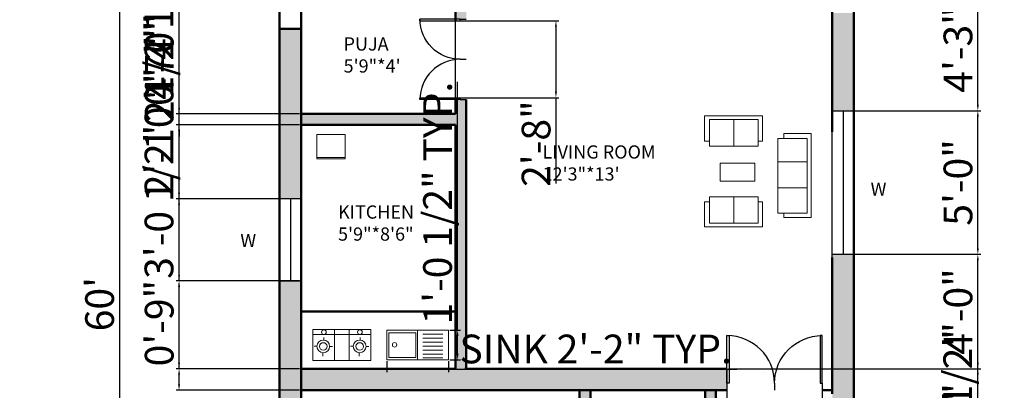
# Model space of a CAD drawing. Units: inches. Extents: x 2063 to 3370, y 2091 to 2971.
# Tile 8 of 14: x 2494 to 2906, y 2468 to 2623. Entities that reach past the tile are written whole.
import ezdxf

# ---------------------------------------------------------------- set-up
doc = ezdxf.new("R2010")
doc.units = ezdxf.units.IN
for name, color, linetype, lineweight in [('A-ANNO-DIMS', 2, 'Continuous', 18), ('A-ANNO-TEXT', 7, 'Continuous', 18), ('A-AREA-IDEN', 3, 'Continuous', 18), ('A-COLS', 7, 'Continuous', 50), ('A-DOOR', 4, 'Continuous', 25), ('A-EQPM', 8, 'Continuous', 18), ('A-FLOR-FIXT', 9, 'Continuous', 18), ('A-FURN', 8, 'Continuous', 18), ('A-GLAZ', 131, 'Continuous', 25), ('A-WALL', 7, 'Continuous', 50), ('A-WALL-PATT', 8, 'Continuous', 13)]:
    doc.layers.add(name, color=color, linetype=linetype, lineweight=lineweight)
doc.styles.get("Standard").update_dxf_attribs({"font": 'arial.ttf'})
doc.dimstyles.new('ISO-25', dxfattribs={"dimtxt": 12, "dimasz": 2.5, "dimexe": 1.25, "dimexo": 0.625, "dimtad": 1, "dimdec": 0, "dimlunit": 4, "dimtxsty": 'Standard', "dimcen": 2.5, "dimadec": 0, "dimazin": 0, "dimtfac": 1, "dimtdec": 0, "dimtmove": 0, "dimatfit": 3, "dimfxl": 1, "dimarcsym": 0})

# ---------------------------------------------------------------- blocks, each defined once
blk = doc.blocks.new('*D8')
at = {"layer": 'A-ANNO-DIMS', "color": 0, "lineweight": -2, "transparency": 16777216}
for p, q in [((2602.12, 2864.43), (2534.59, 2864.43)), ((2535.84, 2861.93), (2535.84, 2146.93)), ((2602.12, 2144.43), (2534.59, 2144.43))]:
    blk.add_line(p, q, dxfattribs=at)
at = {"layer": 'A-ANNO-DIMS', "color": 0, "transparency": 16777216}
for points in [[(2535.42, 2861.93), (2536.25, 2861.93), (2535.84, 2864.43)], [(2535.42, 2146.93), (2536.25, 2146.93), (2535.84, 2144.43)]]:
    blk.add_solid(points, dxfattribs=at)
at = {"layer": 'Defpoints', "color": 0, "transparency": 16777216}
for p in [(2602.75, 2864.43), (2535.84, 2144.43), (2602.75, 2144.43)]:
    blk.add_point(p, dxfattribs=at)
at = {"layer": 'A-ANNO-DIMS', "color": 0, "transparency": 16777216, "insert": (2529.08, 2504.43), "char_height": 12, "attachment_point": 5, "rotation": 90}
blk.add_mtext("60'", dxfattribs=at)
blk = doc.blocks.new('*U2')
for p, q in [((0, 0), (0, -6)), ((40, 0), (40, -6))]:
    blk.add_line(p, q)
blk.add_lwpolyline([(0, 0), (0, 40), (1.75, 40), (1.75, 0)], close=True)
blk.add_arc((0, 0), 40, 0, 90)
blk = doc.blocks.new('SOFA-2SEAT')
for p, q in [((0, 2.07), (0, 12.63)), ((0, 12.63), (24.16, 12.63)), ((24.16, 12.63), (24.16, 2.07)), ((12.27, 11.03), (12.27, 0)), ((2.08, 2.07), (0, 2.07)), ((24.16, 2.07), (22.46, 2.07))]:
    blk.add_line(p, q)
blk.add_lwpolyline([(22.46, 0), (2.08, 0), (2.08, 11.03), (22.46, 11.03)], close=True)
blk = doc.blocks.new('SOFA-3SEAT')
for p, q in [((2.4, 33.13), (2.4, 35.12)), ((2.4, 35.12), (13.91, 35.12)), ((13.91, 35.12), (13.91, 0)), ((0, 23.31), (12.18, 23.31)), ((0, 12.42), (12.18, 12.42)), ((2.4, 0), (2.4, 1.81)), ((13.91, 0), (2.4, 0))]:
    blk.add_line(p, q)
blk.add_lwpolyline([(12.18, 33.13), (0, 33.13), (0, 1.81), (12.18, 1.81)], close=True)
blk = doc.blocks.new('SINK')
for p, q in [((12.88, 12.38), (12.88, 0)), ((15.15, 10.72), (23.41, 10.72)), ((15.15, 9.06), (23.41, 9.06)), ((15.15, 7.39), (23.41, 7.39)), ((15.15, 5.73), (23.41, 5.73)), ((15.15, 4.07), (23.41, 4.07)), ((15.15, 2.41), (23.41, 2.41)), ((15.15, 0.75), (23.41, 0.75))]:
    blk.add_line(p, q)
for points in [[(25.76, 12.38), (0, 12.38), (0, 0), (25.76, 0)], [(0.92, 11.24), (12.1, 11.24), (12.1, 0.97), (0.92, 0.97)]]:
    blk.add_lwpolyline(points, close=True)
blk.add_circle((3.27, 6.25), 0.918)
blk = doc.blocks.new('STOVE')
for p, q in [((0, 12.93), (9.11, 12.93)), ((9.11, 12.93), (9.11, 0)), ((15.17, 0), (15.17, 12.93)), ((0, 10.85), (24.22, 10.85)), ((4.55, 8.54), (4.55, 9.68)), ((19.76, 8.54), (19.76, 9.68)), ((1.72, 5.99), (0.55, 5.99)), ((7.04, 5.79), (8.23, 5.79)), ((16.93, 5.99), (15.75, 5.99)), ((22.25, 5.79), (23.43, 5.79)), ((4.22, 3.16), (4.22, 1.87)), ((24.22, 0), (15.17, 0)), ((19.43, 3.16), (19.43, 1.87))]:
    blk.add_line(p, q)
blk.add_lwpolyline([(0, 12.93), (24.22, 12.93), (24.22, 0), (0, 0)], close=True)
for centre, radius in [((4.62, 11.87), 0.973), ((19.71, 11.87), 0.973), ((4.38, 5.88), 2.66), ((19.59, 5.88), 2.66), ((4.38, 5.88), 1.57), ((19.59, 5.88), 1.57)]:
    blk.add_circle(centre, radius)
blk = doc.blocks.new('*D28')
at = {"layer": 'A-ANNO-DIMS', "color": 0, "lineweight": -2, "transparency": 16777216}
for p, q in [((2647.53, 2480.55), (2647.53, 2476.06)), ((2650.03, 2477.31), (2670.78, 2477.31)), ((2673.28, 2480.55), (2673.28, 2476.06)), ((2673.28, 2477.31), (2793.91, 2477.31))]:
    blk.add_line(p, q, dxfattribs=at)
at = {"layer": 'A-ANNO-DIMS', "color": 0, "transparency": 16777216}
for points in [[(2650.03, 2477.73), (2650.03, 2476.9), (2647.53, 2477.31)], [(2670.78, 2477.73), (2670.78, 2476.9), (2673.28, 2477.31)]]:
    blk.add_solid(points, dxfattribs=at)
at = {"layer": 'Defpoints', "color": 0, "transparency": 16777216}
for p in [(2647.53, 2481.18), (2673.28, 2481.18), (2673.28, 2477.31)]:
    blk.add_point(p, dxfattribs=at)
at = {"layer": 'A-ANNO-DIMS', "color": 0, "transparency": 16777216, "insert": (2734.85, 2484.14), "char_height": 12, "attachment_point": 5}
blk.add_mtext('SINK 2\'-2" TYP.', dxfattribs=at)
blk = doc.blocks.new('*D29')
at = {"layer": 'A-ANNO-DIMS', "color": 0, "lineweight": -2, "transparency": 16777216}
for p, q in [((2677.15, 2493.56), (2677.15, 2597.29)), ((2673.91, 2493.56), (2678.4, 2493.56)), ((2677.15, 2483.68), (2677.15, 2491.06)), ((2673.91, 2481.18), (2678.4, 2481.18))]:
    blk.add_line(p, q, dxfattribs=at)
at = {"layer": 'A-ANNO-DIMS', "color": 0, "transparency": 16777216}
for points in [[(2676.73, 2491.06), (2677.56, 2491.06), (2677.15, 2493.56)], [(2676.73, 2483.68), (2677.56, 2483.68), (2677.15, 2481.18)]]:
    blk.add_solid(points, dxfattribs=at)
at = {"layer": 'Defpoints', "color": 0, "transparency": 16777216}
for p in [(2673.28, 2493.56), (2677.15, 2493.56), (2673.28, 2481.18)]:
    blk.add_point(p, dxfattribs=at)
at = {"layer": 'A-ANNO-DIMS', "color": 0, "transparency": 16777216, "insert": (2670.32, 2546.67), "char_height": 12, "attachment_point": 5, "rotation": 90}
blk.add_mtext('1\'-0 1/2" TYP.', dxfattribs=at)
blk = doc.blocks.new('*D97')
at = {"layer": 'A-ANNO-DIMS', "color": 0, "lineweight": -2, "transparency": 16777216}
for p, q in [((2611.75, 2584.55), (2611.75, 2907.68)), ((2614.25, 2906.43), (2673.75, 2906.43)), ((2676.25, 2584.55), (2676.25, 2907.68))]:
    blk.add_line(p, q, dxfattribs=at)
at = {"layer": 'A-ANNO-DIMS', "color": 0, "transparency": 16777216}
for points in [[(2614.25, 2906.84), (2614.25, 2906.01), (2611.75, 2906.43)], [(2673.75, 2906.84), (2673.75, 2906.01), (2676.25, 2906.43)]]:
    blk.add_solid(points, dxfattribs=at)
at = {"layer": 'Defpoints', "color": 0, "transparency": 16777216}
for p in [(2676.25, 2906.43), (2611.75, 2583.93), (2676.25, 2583.93)]:
    blk.add_point(p, dxfattribs=at)
at = {"layer": 'A-ANNO-DIMS', "color": 0, "transparency": 16777216, "insert": (2644, 2913.26), "char_height": 12, "attachment_point": 5}
blk.add_mtext('5\'-4 1/2"', dxfattribs=at)
blk = doc.blocks.new('*D103')
at = {"layer": 'A-ANNO-DIMS', "color": 0, "lineweight": -2, "transparency": 16777216}
for p, q in [((2560.75, 2477.43), (2560.75, 2513.08)), ((2611.12, 2477.43), (2559.5, 2477.43)), ((2560.75, 2470.93), (2560.75, 2474.93)), ((2611.12, 2468.43), (2559.5, 2468.43))]:
    blk.add_line(p, q, dxfattribs=at)
at = {"layer": 'A-ANNO-DIMS', "color": 0, "transparency": 16777216}
for points in [[(2560.33, 2474.93), (2561.16, 2474.93), (2560.75, 2477.43)], [(2560.33, 2470.93), (2561.16, 2470.93), (2560.75, 2468.43)]]:
    blk.add_solid(points, dxfattribs=at)
at = {"layer": 'Defpoints', "color": 0, "transparency": 16777216}
for p in [(2560.75, 2477.43), (2611.75, 2477.43), (2611.75, 2468.43)]:
    blk.add_point(p, dxfattribs=at)
at = {"layer": 'A-ANNO-DIMS', "color": 0, "transparency": 16777216, "insert": (2554, 2496.5), "char_height": 12, "attachment_point": 5, "rotation": 90}
blk.add_mtext('0\'-9"', dxfattribs=at)
blk = doc.blocks.new('*D104')
at = {"layer": 'A-ANNO-DIMS', "color": 0, "lineweight": -2, "transparency": 16777216}
for p, q in [((2560.75, 2514.15), (2560.75, 2577.75)), ((2611.12, 2514.15), (2559.5, 2514.15)), ((2560.75, 2479.93), (2560.75, 2511.65)), ((2611.12, 2477.43), (2559.5, 2477.43))]:
    blk.add_line(p, q, dxfattribs=at)
at = {"layer": 'A-ANNO-DIMS', "color": 0, "transparency": 16777216}
for points in [[(2560.33, 2511.65), (2561.16, 2511.65), (2560.75, 2514.15)], [(2560.33, 2479.93), (2561.16, 2479.93), (2560.75, 2477.43)]]:
    blk.add_solid(points, dxfattribs=at)
at = {"layer": 'Defpoints', "color": 0, "transparency": 16777216}
for p in [(2560.75, 2514.15), (2611.75, 2514.15), (2611.75, 2477.43)]:
    blk.add_point(p, dxfattribs=at)
at = {"layer": 'A-ANNO-DIMS', "color": 0, "transparency": 16777216, "insert": (2553.91, 2547.2), "char_height": 12, "attachment_point": 5, "rotation": 90}
blk.add_mtext('3\'-0 1/2"', dxfattribs=at)
blk = doc.blocks.new('*D105')
at = {"layer": 'A-ANNO-DIMS', "color": 0, "lineweight": -2, "transparency": 16777216}
for p, q in [((2560.75, 2548.5), (2560.75, 2621.64)), ((2611.12, 2548.5), (2559.5, 2548.5)), ((2560.75, 2516.65), (2560.75, 2546)), ((2611.12, 2514.15), (2559.5, 2514.15))]:
    blk.add_line(p, q, dxfattribs=at)
at = {"layer": 'A-ANNO-DIMS', "color": 0, "transparency": 16777216}
for points in [[(2560.33, 2546), (2561.16, 2546), (2560.75, 2548.5)], [(2560.33, 2516.65), (2561.16, 2516.65), (2560.75, 2514.15)]]:
    blk.add_solid(points, dxfattribs=at)
at = {"layer": 'Defpoints', "color": 0, "transparency": 16777216}
for p in [(2560.75, 2548.5), (2611.75, 2548.5), (2611.75, 2514.15)]:
    blk.add_point(p, dxfattribs=at)
at = {"layer": 'A-ANNO-DIMS', "color": 0, "transparency": 16777216, "insert": (2553.92, 2586.32), "char_height": 12, "attachment_point": 5, "rotation": 90}
blk.add_mtext('2\'-10 1/2"', dxfattribs=at)
blk = doc.blocks.new('*D106')
at = {"layer": 'A-ANNO-DIMS', "color": 0, "lineweight": -2, "transparency": 16777216}
for p, q in [((2560.75, 2579.43), (2560.75, 2615.28)), ((2611.12, 2579.43), (2559.5, 2579.43)), ((2560.75, 2551), (2560.75, 2576.93)), ((2611.12, 2548.5), (2559.5, 2548.5))]:
    blk.add_line(p, q, dxfattribs=at)
at = {"layer": 'A-ANNO-DIMS', "color": 0, "transparency": 16777216}
for points in [[(2560.33, 2576.93), (2561.16, 2576.93), (2560.75, 2579.43)], [(2560.33, 2551), (2561.16, 2551), (2560.75, 2548.5)]]:
    blk.add_solid(points, dxfattribs=at)
at = {"layer": 'Defpoints', "color": 0, "transparency": 16777216}
for p in [(2560.75, 2579.43), (2611.75, 2579.43), (2611.75, 2548.5)]:
    blk.add_point(p, dxfattribs=at)
at = {"layer": 'A-ANNO-DIMS', "color": 0, "transparency": 16777216, "insert": (2554.1, 2598.6), "char_height": 12, "attachment_point": 5, "rotation": 90}
blk.add_mtext('2\'-7"', dxfattribs=at)
blk = doc.blocks.new('*D107')
at = {"layer": 'A-ANNO-DIMS', "color": 0, "lineweight": -2, "transparency": 16777216}
for p, q in [((2560.75, 2586.43), (2560.75, 2650.04)), ((2611.12, 2583.93), (2559.5, 2583.93)), ((2560.75, 2579.43), (2560.75, 2583.93)), ((2611.12, 2579.43), (2559.5, 2579.43)), ((2560.75, 2576.93), (2560.75, 2574.43))]:
    blk.add_line(p, q, dxfattribs=at)
at = {"layer": 'A-ANNO-DIMS', "color": 0, "transparency": 16777216}
for points in [[(2560.33, 2586.43), (2561.16, 2586.43), (2560.75, 2583.93)], [(2560.33, 2576.93), (2561.16, 2576.93), (2560.75, 2579.43)]]:
    blk.add_solid(points, dxfattribs=at)
at = {"layer": 'Defpoints', "color": 0, "transparency": 16777216}
for p in [(2560.75, 2583.93), (2611.75, 2583.93), (2611.75, 2579.43)]:
    blk.add_point(p, dxfattribs=at)
at = {"layer": 'A-ANNO-DIMS', "color": 0, "transparency": 16777216, "insert": (2553.92, 2619.48), "char_height": 12, "attachment_point": 5, "rotation": 90}
blk.add_mtext('0\'-4 1/2"', dxfattribs=at)
blk = doc.blocks.new('*D108')
at = {"layer": 'A-ANNO-DIMS', "color": 0, "lineweight": -2, "transparency": 16777216}
for p, q in [((2611.12, 2631.93), (2559.5, 2631.93)), ((2560.75, 2586.43), (2560.75, 2629.43)), ((2611.12, 2583.93), (2559.5, 2583.93))]:
    blk.add_line(p, q, dxfattribs=at)
at = {"layer": 'A-ANNO-DIMS', "color": 0, "transparency": 16777216}
for points in [[(2560.33, 2629.43), (2561.16, 2629.43), (2560.75, 2631.93)], [(2560.33, 2586.43), (2561.16, 2586.43), (2560.75, 2583.93)]]:
    blk.add_solid(points, dxfattribs=at)
at = {"layer": 'Defpoints', "color": 0, "transparency": 16777216}
for p in [(2560.75, 2631.93), (2611.75, 2631.93), (2611.75, 2583.93)]:
    blk.add_point(p, dxfattribs=at)
at = {"layer": 'A-ANNO-DIMS', "color": 0, "transparency": 16777216, "insert": (2554, 2607.93), "char_height": 12, "attachment_point": 5, "rotation": 90}
blk.add_mtext('4\'-0"', dxfattribs=at)
blk = doc.blocks.new('*D115')
at = {"layer": 'A-ANNO-DIMS', "color": 0, "lineweight": -2, "transparency": 16777216}
for p, q in [((2894.57, 2429.31), (2894.57, 2491.79)), ((2785.76, 2429.31), (2895.82, 2429.31)), ((2894.57, 2416.22), (2894.57, 2426.81)), ((2785.76, 2413.72), (2895.82, 2413.72))]:
    blk.add_line(p, q, dxfattribs=at)
at = {"layer": 'A-ANNO-DIMS', "color": 0, "transparency": 16777216}
for points in [[(2894.15, 2426.81), (2894.99, 2426.81), (2894.57, 2429.31)], [(2894.15, 2416.22), (2894.99, 2416.22), (2894.57, 2413.72)]]:
    blk.add_solid(points, dxfattribs=at)
at = {"layer": 'Defpoints', "color": 0, "transparency": 16777216}
for p in [(2785.14, 2429.31), (2894.57, 2429.31), (2785.14, 2413.72)]:
    blk.add_point(p, dxfattribs=at)
at = {"layer": 'A-ANNO-DIMS', "color": 0, "transparency": 16777216, "insert": (2887.74, 2461.8), "char_height": 12, "attachment_point": 5, "rotation": 90}
blk.add_mtext('1\'-3 1/2"', dxfattribs=at)
blk = doc.blocks.new('*D116')
at = {"layer": 'A-ANNO-DIMS', "color": 0, "lineweight": -2, "transparency": 16777216}
for p, q in [((2790.36, 2477.43), (2895.82, 2477.43)), ((2894.57, 2431.81), (2894.57, 2474.93)), ((2785.76, 2429.31), (2895.82, 2429.31))]:
    blk.add_line(p, q, dxfattribs=at)
at = {"layer": 'A-ANNO-DIMS', "color": 0, "transparency": 16777216}
for points in [[(2894.15, 2474.93), (2894.99, 2474.93), (2894.57, 2477.43)], [(2894.15, 2431.81), (2894.99, 2431.81), (2894.57, 2429.31)]]:
    blk.add_solid(points, dxfattribs=at)
at = {"layer": 'Defpoints', "color": 0, "transparency": 16777216}
for p in [(2789.73, 2477.43), (2894.57, 2477.43), (2785.14, 2429.31)]:
    blk.add_point(p, dxfattribs=at)
at = {"layer": 'A-ANNO-DIMS', "color": 0, "transparency": 16777216, "insert": (2887.82, 2453.37), "char_height": 12, "attachment_point": 5, "rotation": 90}
blk.add_mtext('4\'-0"', dxfattribs=at)
blk = doc.blocks.new('*D117')
at = {"layer": 'A-ANNO-DIMS', "color": 0, "lineweight": -2, "transparency": 16777216}
for p, q in [((2834.37, 2525.28), (2895.82, 2525.28)), ((2894.57, 2479.93), (2894.57, 2522.78)), ((2790.36, 2477.43), (2895.82, 2477.43))]:
    blk.add_line(p, q, dxfattribs=at)
at = {"layer": 'A-ANNO-DIMS', "color": 0, "transparency": 16777216}
for points in [[(2894.15, 2522.78), (2894.99, 2522.78), (2894.57, 2525.28)], [(2894.15, 2479.93), (2894.99, 2479.93), (2894.57, 2477.43)]]:
    blk.add_solid(points, dxfattribs=at)
at = {"layer": 'Defpoints', "color": 0, "transparency": 16777216}
for p in [(2833.75, 2525.28), (2894.57, 2525.28), (2789.73, 2477.43)]:
    blk.add_point(p, dxfattribs=at)
at = {"layer": 'A-ANNO-DIMS', "color": 0, "transparency": 16777216, "insert": (2887.82, 2501.35), "char_height": 12, "attachment_point": 5, "rotation": 90}
blk.add_mtext('4\'-0"', dxfattribs=at)
blk = doc.blocks.new('*D118')
at = {"layer": 'A-ANNO-DIMS', "color": 0, "lineweight": -2, "transparency": 16777216}
for p, q in [((2834.37, 2585.28), (2895.82, 2585.28)), ((2894.57, 2527.78), (2894.57, 2582.78)), ((2834.37, 2525.28), (2895.82, 2525.28))]:
    blk.add_line(p, q, dxfattribs=at)
at = {"layer": 'A-ANNO-DIMS', "color": 0, "transparency": 16777216}
for points in [[(2894.15, 2582.78), (2894.99, 2582.78), (2894.57, 2585.28)], [(2894.15, 2527.78), (2894.99, 2527.78), (2894.57, 2525.28)]]:
    blk.add_solid(points, dxfattribs=at)
at = {"layer": 'Defpoints', "color": 0, "transparency": 16777216}
for p in [(2833.75, 2585.28), (2894.57, 2585.28), (2833.75, 2525.28)]:
    blk.add_point(p, dxfattribs=at)
at = {"layer": 'A-ANNO-DIMS', "color": 0, "transparency": 16777216, "insert": (2887.82, 2555.28), "char_height": 12, "attachment_point": 5, "rotation": 90}
blk.add_mtext('5\'-0"', dxfattribs=at)
blk = doc.blocks.new('*D119')
at = {"layer": 'A-ANNO-DIMS', "color": 0, "lineweight": -2, "transparency": 16777216}
for p, q in [((2834.37, 2636.43), (2895.82, 2636.43)), ((2894.57, 2587.78), (2894.57, 2633.93)), ((2834.37, 2585.28), (2895.82, 2585.28))]:
    blk.add_line(p, q, dxfattribs=at)
at = {"layer": 'A-ANNO-DIMS', "color": 0, "transparency": 16777216}
for points in [[(2894.15, 2633.93), (2894.99, 2633.93), (2894.57, 2636.43)], [(2894.15, 2587.78), (2894.99, 2587.78), (2894.57, 2585.28)]]:
    blk.add_solid(points, dxfattribs=at)
at = {"layer": 'Defpoints', "color": 0, "transparency": 16777216}
for p in [(2833.75, 2636.43), (2894.57, 2636.43), (2833.75, 2585.28)]:
    blk.add_point(p, dxfattribs=at)
at = {"layer": 'A-ANNO-DIMS', "color": 0, "transparency": 16777216, "insert": (2887.82, 2610.85), "char_height": 12, "attachment_point": 5, "rotation": 90}
blk.add_mtext('4\'-3"', dxfattribs=at)
blk = doc.blocks.new('*D130')
at = {"layer": 'A-ANNO-DIMS', "color": 0, "lineweight": -2, "transparency": 16777216}
for p, q in [((2676.87, 2622.85), (2719.5, 2622.85)), ((2718.25, 2620.35), (2718.25, 2593.19)), ((2676.87, 2590.69), (2719.5, 2590.69)), ((2718.25, 2590.69), (2718.25, 2554.84))]:
    blk.add_line(p, q, dxfattribs=at)
at = {"layer": 'A-ANNO-DIMS', "color": 0, "transparency": 16777216}
for points in [[(2717.83, 2620.35), (2718.66, 2620.35), (2718.25, 2622.85)], [(2717.83, 2593.19), (2718.66, 2593.19), (2718.25, 2590.69)]]:
    blk.add_solid(points, dxfattribs=at)
at = {"layer": 'Defpoints', "color": 0, "transparency": 16777216}
for p in [(2676.25, 2622.85), (2676.25, 2590.69), (2718.25, 2590.69)]:
    blk.add_point(p, dxfattribs=at)
at = {"layer": 'A-ANNO-DIMS', "color": 0, "transparency": 16777216, "insert": (2711.5, 2571.52), "char_height": 12, "attachment_point": 5, "rotation": 90}
blk.add_mtext('2\'-8"', dxfattribs=at)
blk = doc.blocks.new('*D131')
at = {"layer": 'A-ANNO-DIMS', "color": 0, "lineweight": -2, "transparency": 16777216}
for p, q in [((2789.73, 2476.8), (2789.73, 2101.18)), ((2829.49, 2470.78), (2829.49, 2101.18)), ((2792.23, 2102.43), (2826.99, 2102.43))]:
    blk.add_line(p, q, dxfattribs=at)
at = {"layer": 'A-ANNO-DIMS', "color": 0, "transparency": 16777216}
for points in [[(2792.23, 2102.84), (2792.23, 2102.01), (2789.73, 2102.43)], [(2826.99, 2102.84), (2826.99, 2102.01), (2829.49, 2102.43)]]:
    blk.add_solid(points, dxfattribs=at)
at = {"layer": 'Defpoints', "color": 0, "transparency": 16777216}
for p in [(2789.73, 2477.43), (2829.49, 2471.41), (2829.49, 2102.43)]:
    blk.add_point(p, dxfattribs=at)
at = {"layer": 'A-ANNO-DIMS', "color": 0, "transparency": 16777216, "insert": (2809.61, 2109.18), "char_height": 12, "attachment_point": 5}
blk.add_mtext('3\'-4"', dxfattribs=at)

msp = doc.modelspace()

# ---------------------------------------------------------------- hatches: boundary and pattern name
at = {"layer": 'A-WALL-PATT'}
h = msp.add_hatch(color=256, dxfattribs=at)
h.dxf.hatch_style = 1
h.paths.add_polyline_path([(2842.75, 2864.43), (2602.75, 2864.43), (2602.75, 2831.43), (2608.62, 2831.43), (2608.62, 2859.54), (2836.36, 2859.54), (2836.36, 2831.15), (2842.75, 2831.15)])
h.paths.add_polyline_path([(2775.49, 2177.04), (2815.13, 2177.04), (2815.13, 2197.65), (2775.49, 2197.65)], flags=9)
h.paths.add_polyline_path([(2634.18, 2285.75), (2670.81, 2285.75), (2670.81, 2306.35), (2634.18, 2306.35)], flags=9)
h.paths.add_polyline_path([(2701.65, 2293.1), (2755.85, 2293.1), (2755.85, 2313.71), (2701.65, 2313.71)], flags=9)
h.paths.add_polyline_path([(2735.8, 2415.55), (2772.95, 2415.55), (2772.95, 2436.13), (2735.8, 2436.13)], flags=9)
h.paths.add_polyline_path([(2641.75, 2422.21), (2718.67, 2422.21), (2718.67, 2442.82), (2641.75, 2442.82)], flags=9)
h.paths.add_polyline_path([(2710.43, 2552.92), (2764.91, 2552.92), (2764.91, 2573.53), (2710.43, 2573.53)], flags=9)
h.paths.add_polyline_path([(2625.23, 2527.83), (2661.86, 2527.83), (2661.86, 2548.44), (2625.23, 2548.44)], flags=9)
h.paths.add_polyline_path([(2627.53, 2598.16), (2652.13, 2598.16), (2652.13, 2618.77), (2627.53, 2618.77)], flags=9)
h.paths.add_polyline_path([(2646.64, 2696.08), (2723.56, 2696.08), (2723.56, 2716.69), (2646.64, 2716.69)], flags=9)
h.paths.add_polyline_path([(2791.65, 2795.64), (2828.72, 2795.64), (2828.72, 2807.02), (2791.65, 2807.02)], flags=9)
h.paths.add_polyline_path([(2751.88, 2214.78), (2761.93, 2214.78), (2761.93, 2226.17), (2751.88, 2226.17)], flags=9)
h.paths.add_polyline_path([(2664.96, 2215.71), (2675, 2215.71), (2675, 2227.09), (2664.96, 2227.09)], flags=9)
h.paths.add_polyline_path([(2788.26, 2413.43), (2796.17, 2413.43), (2796.17, 2424.82), (2788.26, 2424.82)], flags=9)
h.paths.add_polyline_path([(2728.86, 2795.64), (2765.93, 2795.64), (2765.93, 2807.02), (2728.86, 2807.02)], flags=9)
h.paths.add_polyline_path([(2760.39, 2726.09), (2823.16, 2726.09), (2823.16, 2746.7), (2760.39, 2746.7)], flags=9)
h = msp.add_hatch(color=256, dxfattribs=at)
h.dxf.hatch_style = 1
h.paths.add_polyline_path([(2290.22, 2192.43), (2278.22, 2192.43), (2182.22, 2192.43), (2182.22, 2189.43), (2182.22, 2187.43), (2278.22, 2187.43), (2290.22, 2187.42)])
h.paths.add_polyline_path([(2748.25, 2192.43), (2736.25, 2192.43), (2640.25, 2192.43), (2640.25, 2189.43), (2640.25, 2187.43), (2736.25, 2187.43), (2748.25, 2187.42)], flags=17)
h.paths.add_polyline_path([(2653.66, 2234.43), (2611.75, 2234.43), (2611.75, 2232.93), (2611.75, 2225.43), (2653.66, 2225.43)])
h.paths.add_polyline_path([(2717.13, 2234.43), (2675.81, 2234.43), (2675.81, 2225.43), (2717.13, 2225.43)])
h.paths.add_polyline_path([(2611.75, 2222.57), (2602.75, 2222.57), (2602.75, 2144.43), (2842.75, 2144.43), (2842.75, 2220.3), (2833.75, 2220.3), (2833.75, 2153.43), (2829.39, 2153.43), (2754.78, 2153.43), (2611.75, 2153.43)])
h.paths.add_polyline_path([(2687.64, 2308.91), (2683.14, 2308.91), (2683.14, 2234.43), (2687.64, 2234.43)])
h.paths.add_polyline_path([(2744.5, 2234.43), (2736.25, 2234.43), (2736.25, 2225.43), (2744.5, 2225.43)])
h.paths.add_polyline_path([(2785.14, 2260.02), (2782.31, 2260.02), (2780.64, 2260.02), (2780.64, 2234.43), (2766.65, 2234.43), (2766.65, 2225.43), (2785.14, 2225.43)])
h.paths.add_polyline_path([(2842.75, 2363.93), (2833.75, 2363.93), (2833.75, 2239.41), (2842.75, 2239.41)])
h.paths.add_polyline_path([(2775.49, 2177.04), (2815.13, 2177.04), (2815.13, 2197.65), (2775.49, 2197.65)], flags=25)
h.paths.add_polyline_path([(2634.18, 2285.75), (2670.81, 2285.75), (2670.81, 2306.35), (2634.18, 2306.35)], flags=9)
h.paths.add_polyline_path([(2701.65, 2293.1), (2755.85, 2293.1), (2755.85, 2313.71), (2701.65, 2313.71)], flags=9)
h.paths.add_polyline_path([(2735.8, 2415.55), (2772.95, 2415.55), (2772.95, 2436.13), (2735.8, 2436.13)], flags=9)
h.paths.add_polyline_path([(2641.75, 2422.21), (2718.67, 2422.21), (2718.67, 2442.82), (2641.75, 2442.82)], flags=9)
h.paths.add_polyline_path([(2710.43, 2552.92), (2764.91, 2552.92), (2764.91, 2573.53), (2710.43, 2573.53)], flags=9)
h.paths.add_polyline_path([(2625.23, 2527.83), (2661.86, 2527.83), (2661.86, 2548.44), (2625.23, 2548.44)], flags=9)
h.paths.add_polyline_path([(2627.53, 2598.16), (2652.13, 2598.16), (2652.13, 2618.77), (2627.53, 2618.77)], flags=9)
h.paths.add_polyline_path([(2646.64, 2696.08), (2723.56, 2696.08), (2723.56, 2716.69), (2646.64, 2716.69)], flags=9)
h.paths.add_polyline_path([(2791.65, 2795.64), (2828.72, 2795.64), (2828.72, 2807.02), (2791.65, 2807.02)], flags=9)
h.paths.add_polyline_path([(2751.88, 2214.78), (2761.93, 2214.78), (2761.93, 2226.17), (2751.88, 2226.17)], flags=9)
h.paths.add_polyline_path([(2788.26, 2413.43), (2796.17, 2413.43), (2796.17, 2424.82), (2788.26, 2424.82)], flags=9)
h.paths.add_polyline_path([(2761.97, 2835.24), (2769.88, 2835.24), (2769.88, 2846.62), (2761.97, 2846.62)], flags=9)
h.paths.add_polyline_path([(2675.89, 2833.68), (2685.93, 2833.68), (2685.93, 2845.06), (2675.89, 2845.06)], flags=9)
h.paths.add_polyline_path([(2728.86, 2795.64), (2765.93, 2795.64), (2765.93, 2807.02), (2728.86, 2807.02)], flags=9)
h.paths.add_polyline_path([(2760.39, 2726.09), (2823.16, 2726.09), (2823.16, 2746.7), (2760.39, 2746.7)], flags=9)
h = msp.add_hatch(color=256, dxfattribs=at)
h.dxf.hatch_style = 1
h.paths.add_polyline_path([(2680.75, 2631.93), (2684.44, 2631.93), (2684.44, 2636.43), (2683.1, 2636.43), (2611.75, 2636.43), (2611.75, 2631.93), (2648.72, 2631.93), (2671.75, 2631.93), (2676.25, 2631.93), (2676.25, 2623.58), (2678.23, 2623.58), (2680.75, 2623.58)])
h.paths.add_polyline_path([(2728.75, 2636.43), (2724.44, 2636.43), (2724.44, 2631.93), (2728.75, 2631.93)])
h.paths.add_polyline_path([(2772.02, 2636.43), (2733.25, 2636.43), (2733.25, 2631.93), (2772.02, 2631.93)])
h.paths.add_polyline_path([(2733.25, 2636.43), (2728.75, 2636.43), (2728.75, 2631.93), (2733.25, 2631.93)])
h.paths.add_polyline_path([(2833.75, 2636.43), (2812.02, 2636.43), (2812.02, 2631.93), (2833.75, 2631.93)])
h.paths.add_polyline_path([(2842.75, 2626.16), (2833.75, 2626.16), (2833.75, 2585.28), (2842.75, 2585.28)])
h.paths.add_polyline_path([(2842.75, 2679.03), (2833.75, 2679.03), (2833.75, 2645.28), (2842.75, 2645.28)])
h.paths.add_polyline_path([(2611.75, 2619.52), (2602.75, 2619.52), (2602.75, 2548.5), (2611.75, 2548.5), (2611.75, 2579.43)])
h.paths.add_polyline_path([(2646.64, 2696.08), (2723.56, 2696.08), (2723.56, 2716.69), (2646.64, 2716.69)], flags=9)
h.paths.add_polyline_path([(2791.65, 2795.64), (2828.72, 2795.64), (2828.72, 2807.02), (2791.65, 2807.02)], flags=9)
h.paths.add_polyline_path([(2761.97, 2835.24), (2769.88, 2835.24), (2769.88, 2846.62), (2761.97, 2846.62)], flags=9)
h.paths.add_polyline_path([(2675.89, 2833.68), (2685.93, 2833.68), (2685.93, 2845.06), (2675.89, 2845.06)], flags=9)
h.paths.add_polyline_path([(2728.86, 2795.64), (2765.93, 2795.64), (2765.93, 2807.02), (2728.86, 2807.02)], flags=9)
h.paths.add_polyline_path([(2775.49, 2177.04), (2815.13, 2177.04), (2815.13, 2197.65), (2775.49, 2197.65)], flags=9)
h.paths.add_polyline_path([(2634.18, 2285.75), (2670.81, 2285.75), (2670.81, 2306.35), (2634.18, 2306.35)], flags=9)
h.paths.add_polyline_path([(2701.65, 2293.1), (2755.85, 2293.1), (2755.85, 2313.71), (2701.65, 2313.71)], flags=9)
h.paths.add_polyline_path([(2735.8, 2415.55), (2772.95, 2415.55), (2772.95, 2436.13), (2735.8, 2436.13)], flags=9)
h.paths.add_polyline_path([(2641.75, 2422.21), (2718.67, 2422.21), (2718.67, 2442.82), (2641.75, 2442.82)], flags=9)
h.paths.add_polyline_path([(2710.43, 2552.92), (2764.91, 2552.92), (2764.91, 2573.53), (2710.43, 2573.53)], flags=9)
h.paths.add_polyline_path([(2625.23, 2527.83), (2661.86, 2527.83), (2661.86, 2548.44), (2625.23, 2548.44)], flags=9)
h.paths.add_polyline_path([(2751.88, 2214.78), (2761.93, 2214.78), (2761.93, 2226.17), (2751.88, 2226.17)], flags=9)
h.paths.add_polyline_path([(2664.96, 2215.71), (2675, 2215.71), (2675, 2227.09), (2664.96, 2227.09)], flags=9)
h.paths.add_polyline_path([(2788.26, 2413.43), (2796.17, 2413.43), (2796.17, 2424.82), (2788.26, 2424.82)], flags=9)
h = msp.add_hatch(color=256, dxfattribs=at)
h.dxf.hatch_style = 1
h.paths.add_polyline_path([(2611.75, 2343.93), (2611.75, 2477.43), (2611.75, 2514.15), (2602.75, 2514.15), (2602.75, 2241.68), (2611.75, 2241.68), (2611.75, 2258.43)])
h.paths.add_polyline_path([(2775.49, 2177.04), (2815.13, 2177.04), (2815.13, 2197.65), (2775.49, 2197.65)], flags=9)
h.paths.add_polyline_path([(2735.8, 2415.55), (2772.95, 2415.55), (2772.95, 2436.13), (2735.8, 2436.13)], flags=9)
h.paths.add_polyline_path([(2641.75, 2422.21), (2718.67, 2422.21), (2718.67, 2442.82), (2641.75, 2442.82)], flags=9)
h.paths.add_polyline_path([(2710.43, 2552.92), (2764.91, 2552.92), (2764.91, 2573.53), (2710.43, 2573.53)], flags=9)
h.paths.add_polyline_path([(2625.23, 2527.83), (2661.86, 2527.83), (2661.86, 2548.44), (2625.23, 2548.44)], flags=9)
h.paths.add_polyline_path([(2627.53, 2598.16), (2652.13, 2598.16), (2652.13, 2618.77), (2627.53, 2618.77)], flags=9)
h.paths.add_polyline_path([(2646.64, 2696.08), (2723.56, 2696.08), (2723.56, 2716.69), (2646.64, 2716.69)], flags=9)
h.paths.add_polyline_path([(2791.65, 2795.64), (2828.72, 2795.64), (2828.72, 2807.02), (2791.65, 2807.02)], flags=9)
h.paths.add_polyline_path([(2751.88, 2214.78), (2761.93, 2214.78), (2761.93, 2226.17), (2751.88, 2226.17)], flags=9)
h.paths.add_polyline_path([(2788.26, 2413.43), (2796.17, 2413.43), (2796.17, 2424.82), (2788.26, 2424.82)], flags=9)
h.paths.add_polyline_path([(2761.97, 2835.24), (2769.88, 2835.24), (2769.88, 2846.62), (2761.97, 2846.62)], flags=9)
h.paths.add_polyline_path([(2675.89, 2833.68), (2685.93, 2833.68), (2685.93, 2845.06), (2675.89, 2845.06)], flags=9)
h.paths.add_polyline_path([(2728.86, 2795.64), (2765.93, 2795.64), (2765.93, 2807.02), (2728.86, 2807.02)], flags=9)
h.paths.add_polyline_path([(2760.39, 2726.09), (2823.16, 2726.09), (2823.16, 2746.7), (2760.39, 2746.7)], flags=9)
h = msp.add_hatch(color=256, dxfattribs=at)
h.dxf.hatch_style = 1
h.paths.add_polyline_path([(2785.14, 2468.43), (2780.64, 2468.43), (2780.64, 2429.31), (2785.14, 2429.31)])
h.paths.add_polyline_path([(2842.75, 2525.28), (2833.75, 2525.28), (2833.75, 2523.93), (2833.75, 2466.93), (2833.75, 2383.04), (2842.75, 2383.04)])
h.paths.add_polyline_path([(2789.73, 2477.43), (2680.75, 2477.43), (2680.75, 2579.43), (2680.75, 2589.96), (2678.23, 2589.96), (2676.25, 2589.96), (2676.25, 2583.93), (2667.25, 2583.93), (2611.75, 2583.93), (2611.75, 2579.43), (2671.75, 2579.43), (2676.25, 2579.43), (2676.25, 2477.43), (2611.75, 2477.43), (2611.75, 2468.43), (2728.75, 2468.43), (2789.73, 2468.43), (2789.73, 2471.41)])
h.paths.add_polyline_path([(2710.43, 2552.92), (2764.91, 2552.92), (2764.91, 2573.53), (2710.43, 2573.53)], flags=25)
h.paths.add_polyline_path([(2625.23, 2527.83), (2661.86, 2527.83), (2661.86, 2548.44), (2625.23, 2548.44)], flags=25)
h.paths.add_polyline_path([(2627.53, 2598.16), (2652.13, 2598.16), (2652.13, 2618.77), (2627.53, 2618.77)], flags=9)
h.paths.add_polyline_path([(2646.64, 2696.08), (2723.56, 2696.08), (2723.56, 2716.69), (2646.64, 2716.69)], flags=9)
h.paths.add_polyline_path([(2791.65, 2795.64), (2828.72, 2795.64), (2828.72, 2807.02), (2791.65, 2807.02)], flags=9)
h.paths.add_polyline_path([(2761.97, 2835.24), (2769.88, 2835.24), (2769.88, 2846.62), (2761.97, 2846.62)], flags=9)
h.paths.add_polyline_path([(2675.89, 2833.68), (2685.93, 2833.68), (2685.93, 2845.06), (2675.89, 2845.06)], flags=9)
h.paths.add_polyline_path([(2728.86, 2795.64), (2765.93, 2795.64), (2765.93, 2807.02), (2728.86, 2807.02)], flags=9)
h.paths.add_polyline_path([(2760.39, 2726.09), (2823.16, 2726.09), (2823.16, 2746.7), (2760.39, 2746.7)], flags=9)
h.paths.add_polyline_path([(2775.49, 2177.04), (2815.13, 2177.04), (2815.13, 2197.65), (2775.49, 2197.65)], flags=9)
h.paths.add_polyline_path([(2634.18, 2285.75), (2670.81, 2285.75), (2670.81, 2306.35), (2634.18, 2306.35)], flags=9)
h.paths.add_polyline_path([(2701.65, 2293.1), (2755.85, 2293.1), (2755.85, 2313.71), (2701.65, 2313.71)], flags=9)
h.paths.add_polyline_path([(2641.75, 2422.21), (2718.67, 2422.21), (2718.67, 2442.82), (2641.75, 2442.82)], flags=9)
h.paths.add_polyline_path([(2751.88, 2214.78), (2761.93, 2214.78), (2761.93, 2226.17), (2751.88, 2226.17)], flags=9)
h.paths.add_polyline_path([(2664.96, 2215.71), (2675, 2215.71), (2675, 2227.09), (2664.96, 2227.09)], flags=9)
h.paths.add_polyline_path([(2788.26, 2413.43), (2796.17, 2413.43), (2796.17, 2424.82), (2788.26, 2424.82)], flags=9)
h = msp.add_hatch(color=256, dxfattribs=at)
h.dxf.hatch_style = 1
h.paths.add_polyline_path([(2785.14, 2343.93), (2785.14, 2392.49), (2785.14, 2413.72), (2780.64, 2413.72), (2780.64, 2384.43), (2780.64, 2348.43), (2732.64, 2348.43), (2732.64, 2360.22), (2728.14, 2360.22), (2728.14, 2348.43), (2725.61, 2348.43), (2725.61, 2348.17), (2725.61, 2343.93), (2780.64, 2343.93), (2780.64, 2329.91), (2780.64, 2297.78), (2782.31, 2297.78), (2785.14, 2297.78)])
h.paths.add_polyline_path([(2732.64, 2396.29), (2731.36, 2396.29), (2728.14, 2396.29), (2728.14, 2379.34), (2732.64, 2379.34)], flags=17)
h.paths.add_polyline_path([(2732.64, 2468.43), (2728.14, 2468.43), (2728.14, 2417.8), (2731.36, 2417.8, -0.014809), (2732.64, 2417.76)])
h.paths.add_polyline_path([(2697.29, 2348.43), (2611.75, 2348.43), (2611.75, 2343.93), (2683.14, 2343.93), (2697.29, 2343.93)])
h.paths.add_polyline_path([(2710.43, 2552.92), (2764.91, 2552.92), (2764.91, 2573.53), (2710.43, 2573.53)], flags=9)
h.paths.add_polyline_path([(2625.23, 2527.83), (2661.86, 2527.83), (2661.86, 2548.44), (2625.23, 2548.44)], flags=9)
h.paths.add_polyline_path([(2627.53, 2598.16), (2652.13, 2598.16), (2652.13, 2618.77), (2627.53, 2618.77)], flags=9)
h.paths.add_polyline_path([(2646.64, 2696.08), (2723.56, 2696.08), (2723.56, 2716.69), (2646.64, 2716.69)], flags=9)
h.paths.add_polyline_path([(2791.65, 2795.64), (2828.72, 2795.64), (2828.72, 2807.02), (2791.65, 2807.02)], flags=9)
h.paths.add_polyline_path([(2761.97, 2835.24), (2769.88, 2835.24), (2769.88, 2846.62), (2761.97, 2846.62)], flags=9)
h.paths.add_polyline_path([(2675.89, 2833.68), (2685.93, 2833.68), (2685.93, 2845.06), (2675.89, 2845.06)], flags=9)
h.paths.add_polyline_path([(2728.86, 2795.64), (2765.93, 2795.64), (2765.93, 2807.02), (2728.86, 2807.02)], flags=9)
h.paths.add_polyline_path([(2760.39, 2726.09), (2823.16, 2726.09), (2823.16, 2746.7), (2760.39, 2746.7)], flags=9)
h = msp.add_hatch(color=256, dxfattribs=at)
h.dxf.hatch_style = 1
h.paths.add_polyline_path([(2655.27, 2831.43), (2611.75, 2831.43), (2611.75, 2822.43), (2655.27, 2822.43)])
h.paths.add_polyline_path([(2722.06, 2831.43), (2703.27, 2831.43), (2703.27, 2822.43), (2722.06, 2822.43)])
h.paths.add_polyline_path([(2754.66, 2831.43), (2741.18, 2831.43), (2741.18, 2822.43), (2754.66, 2822.43)])
h.paths.add_polyline_path([(2833.75, 2831.43), (2779.09, 2831.43), (2779.09, 2822.43), (2833.75, 2822.43)])
h.paths.add_polyline_path([(2790.07, 2822.43), (2785.57, 2822.43), (2785.57, 2774.43), (2790.07, 2774.43)])
h.paths.add_polyline_path([(2775.49, 2177.04), (2815.13, 2177.04), (2815.13, 2197.65), (2775.49, 2197.65)], flags=9)
h.paths.add_polyline_path([(2634.18, 2285.75), (2670.81, 2285.75), (2670.81, 2306.35), (2634.18, 2306.35)], flags=9)
h.paths.add_polyline_path([(2701.65, 2293.1), (2755.85, 2293.1), (2755.85, 2313.71), (2701.65, 2313.71)], flags=9)
h.paths.add_polyline_path([(2735.8, 2415.55), (2772.95, 2415.55), (2772.95, 2436.13), (2735.8, 2436.13)], flags=9)
h.paths.add_polyline_path([(2641.75, 2422.21), (2718.67, 2422.21), (2718.67, 2442.82), (2641.75, 2442.82)], flags=9)
h.paths.add_polyline_path([(2710.43, 2552.92), (2764.91, 2552.92), (2764.91, 2573.53), (2710.43, 2573.53)], flags=9)
h.paths.add_polyline_path([(2625.23, 2527.83), (2661.86, 2527.83), (2661.86, 2548.44), (2625.23, 2548.44)], flags=9)
h.paths.add_polyline_path([(2627.53, 2598.16), (2652.13, 2598.16), (2652.13, 2618.77), (2627.53, 2618.77)], flags=9)
h.paths.add_polyline_path([(2646.64, 2696.08), (2723.56, 2696.08), (2723.56, 2716.69), (2646.64, 2716.69)], flags=9)
h.paths.add_polyline_path([(2791.65, 2795.64), (2828.72, 2795.64), (2828.72, 2807.02), (2791.65, 2807.02)], flags=9)
h.paths.add_polyline_path([(2751.88, 2214.78), (2761.93, 2214.78), (2761.93, 2226.17), (2751.88, 2226.17)], flags=9)
h.paths.add_polyline_path([(2664.96, 2215.71), (2675, 2215.71), (2675, 2227.09), (2664.96, 2227.09)], flags=9)
h.paths.add_polyline_path([(2788.26, 2413.43), (2796.17, 2413.43), (2796.17, 2424.82), (2788.26, 2424.82)], flags=9)
h.paths.add_polyline_path([(2728.86, 2795.64), (2765.93, 2795.64), (2765.93, 2807.02), (2728.86, 2807.02)], flags=9)
h.paths.add_polyline_path([(2760.39, 2726.09), (2823.16, 2726.09), (2823.16, 2746.7), (2760.39, 2746.7)], flags=9)

# ---------------------------------------------------------------- linework, layer by layer
at = {"layer": 'A-COLS'}
msp.add_lwpolyline([(2602.75, 2638.63), (2611.75, 2638.63), (2611.75, 2619.52), (2602.75, 2619.52)], close=True, dxfattribs=at)
at = {"layer": 'A-EQPM'}
msp.add_line((2618.35, 2565.71), (2630.17, 2565.71), dxfattribs=at)
msp.add_lwpolyline([(2618.35, 2575.31), (2630.17, 2575.31), (2630.17, 2565.19), (2618.35, 2565.19)], close=True, dxfattribs=at)
at = {"layer": 'A-FURN'}
msp.add_lwpolyline([(2786.9, 2563.33), (2801.38, 2563.33), (2801.38, 2555.77), (2786.9, 2555.77)], close=True, dxfattribs=at)
at = {"layer": 'A-GLAZ'}
for p, q in [((2833.75, 2528.28), (2833.75, 2585.28)), ((2833.75, 2585.28), (2842.75, 2585.28)), ((2838.25, 2585.28), (2838.25, 2525.28)), ((2607.25, 2548.5), (2607.25, 2514.15)), ((2833.75, 2525.28), (2842.75, 2525.28))]:
    msp.add_line(p, q, dxfattribs=at)
for points in [[(2833.75, 2532.78), (2833.75, 2580.78)], [(2833.75, 2523.93), (2833.75, 2571.93)]]:
    msp.add_lwpolyline(points, dxfattribs=at)
msp.add_lwpolyline([(2611.75, 2548.5), (2602.75, 2548.5), (2602.75, 2514.15), (2611.75, 2514.15)], close=True, dxfattribs=at)
at = {"layer": 'A-WALL'}
for p, q in [((2676.25, 2622.85), (2676.25, 2631.93)), ((2676.25, 2583.93), (2676.25, 2590.69)), ((2680.75, 2579.43), (2680.75, 2589.96)), ((2611.75, 2583.93), (2671.75, 2583.93)), ((2667.25, 2583.93), (2676.25, 2583.93)), ((2611.75, 2579.43), (2671.75, 2579.43)), ((2611.75, 2579.43), (2611.75, 2477.43)), ((2676.25, 2579.43), (2667.28, 2579.43)), ((2676.25, 2477.43), (2676.25, 2579.43)), ((2680.75, 2477.43), (2680.75, 2579.43)), ((2833.75, 2466.93), (2833.75, 2523.93)), ((2611.75, 2477.43), (2611.8, 2501.43)), ((2611.8, 2501.43), (2676.25, 2501.43)), ((2611.75, 2477.43), (2676.25, 2477.43)), ((2611.75, 2477.43), (2676.25, 2477.43)), ((2611.75, 2241.68), (2611.75, 2477.43)), ((2680.14, 2477.43), (2732.64, 2477.43)), ((2680.75, 2477.43), (2789.73, 2477.43)), ((2732.64, 2477.43), (2785.14, 2477.43)), ((2805.27, 2476.04), (2805.27, 2476.04)), ((2611.75, 2468.43), (2680.75, 2468.43)), ((2611.75, 2468.43), (2728.75, 2468.43)), ((2611.75, 2468.43), (2611.75, 2348.43)), ((2680.75, 2468.43), (2789.73, 2468.43)), ((2728.14, 2468.43), (2728.14, 2417.8)), ((2732.64, 2468.43), (2732.64, 2417.76)), ((2732.64, 2468.43), (2780.64, 2468.43)), ((2780.64, 2468.43), (2780.64, 2384.43)), ((2785.14, 2468.43), (2785.14, 2384.43)), ((2829.49, 2468.43), (2833.75, 2468.43))]:
    msp.add_line(p, q, dxfattribs=at)
msp.add_lwpolyline([(2602.75, 2144.43), (2842.75, 2144.43), (2842.75, 2864.43), (2602.75, 2864.43)], close=True, dxfattribs=at)
for points in [[(2611.75, 2822.43), (2611.75, 2576.43)], [(2833.75, 2576.43), (2833.75, 2769.93)], [(2611.75, 2631.93), (2611.75, 2583.93)], [(2611.75, 2579.43), (2611.75, 2531.43)], [(2833.75, 2471.43), (2833.75, 2519.43)]]:
    msp.add_lwpolyline(points, dxfattribs=at)

# ---------------------------------------------------------------- block references
at = {"layer": 'A-DOOR', "yscale": 0.4203428619043682, "zscale": 0.4203428619043682, "rotation": 90}
for p, xscale in [((2678.23, 2623.58), -0.4203428619043682), ((2678.23, 2589.96), 0.4203428619043682)]:
    msp.add_blockref('*U2', p, dxfattribs=dict(at, xscale=xscale))
at = {"layer": 'A-DOOR', "yscale": 0.4970278449321303, "zscale": 0.4970278449321303}
for p, xscale in [((2789.73, 2471.41), 0.4970278449321303), ((2829.49, 2471.41), -0.4970278449321303)]:
    msp.add_blockref('*U2', p, dxfattribs=dict(at, xscale=xscale))
at = {"layer": 'A-FLOR-FIXT'}
for name, p in [('STOVE', (2616.64, 2480.88)), ('SINK', (2647.53, 2481.18))]:
    msp.add_blockref(name, p, dxfattribs=at)
at = {"layer": 'A-FURN'}
for name, p in [('SOFA-2SEAT', (2780.37, 2570.52)), ('SOFA-3SEAT', (2811.04, 2540.59))]:
    msp.add_blockref(name, p, dxfattribs=at)
at = {"layer": 'A-FURN', "extrusion": (0, 0, -1), "zscale": -1, "rotation": 180}
msp.add_blockref('SOFA-2SEAT', (-2780.37, 2549.32), dxfattribs=at)

# ---------------------------------------------------------------- texts
at = {"layer": 'A-ANNO-TEXT', "char_height": 5.52, "attachment_point": 1}
for insert in [(2849.75, 2555.25), (2586.34, 2533.8)]:
    msp.add_mtext_dynamic_manual_height_columns('W', width=106.0361, gutter_width=27.61, heights=[0], dxfattribs=dict(at, insert=insert))
at = {"layer": 'A-AREA-IDEN', "attachment_point": 1}
for s, heights, insert, char_height in [('PUJA \\P5\'9"*4\'', [14.84], (2629.5, 2615.93), 5.523), ('LIVING ROOM\\P12\'3"*13\'', [0], (2712.65, 2570.79), 5.5229), ('KITCHEN\\P5\'9"*8\'6"', [0], (2627.18, 2545.69), 5.523)]:
    msp.add_mtext_dynamic_manual_height_columns(s, width=106.0361, gutter_width=27.61, heights=heights, dxfattribs=dict(at, insert=insert, char_height=char_height))

# ---------------------------------------------------------------- dimensions: what is measured, and where the dimension line sits
at = {"layer": 'A-ANNO-DIMS'}
for base, p1, p2, picture, middle in [((2676.25, 2906.43), (2611.75, 2583.93), (2676.25, 2583.93), '*D97', (2644, 2913.26)), ((2829.49, 2102.43), (2789.73, 2477.43), (2829.49, 2471.41), '*D131', (2809.61, 2109.18))]:
    dim = msp.add_linear_dim(base=base, p1=p1, p2=p2, dimstyle='ISO-25', override={"dimdec": 1, "dimlfac": 1, "dimrnd": 0, "dimzin": 1, "dimdsep": 46, "dimlunit": 4, "dimfrac": 2}, dxfattribs=at)
    dim.commit()
    dim.dimension.update_dxf_attribs({"geometry": picture, "text_midpoint": middle})
for base, p1, p2, angle, override, picture, middle in [((2535.84, 2144.43), (2602.75, 2864.43), (2602.75, 2144.43), 90, {"dimclrd": 0, "dimclre": 0, "dimclrt": 0}, '*D8', (2529.08, 2504.43)), ((2560.75, 2583.93), (2611.75, 2579.43), (2611.75, 2583.93), 90, {"dimdec": 1, "dimlfac": 1, "dimrnd": 0, "dimzin": 1, "dimdsep": 46, "dimlunit": 4, "dimfrac": 2}, '*D107', (2553.92, 2619.48)), ((2894.5713, 2636.4264), (2833.7472, 2585.2786), (2833.7472, 2636.4264), 90, {"dimdec": 1, "dimlfac": 1, "dimrnd": 0, "dimzin": 1, "dimdsep": 46, "dimlunit": 4, "dimfrac": 2}, '*D119', (2887.8154, 2610.8525)), ((2560.75, 2631.93), (2611.75, 2583.93), (2611.75, 2631.93), 90, {"dimdec": 1, "dimlfac": 1, "dimrnd": 0, "dimzin": 1, "dimdsep": 46, "dimlunit": 4, "dimfrac": 2}, '*D108', (2554, 2607.93)), ((2560.7472, 2548.4974), (2611.7472, 2514.1508), (2611.7472, 2548.4974), 90, {"dimdec": 1, "dimlfac": 1, "dimrnd": 0, "dimzin": 1, "dimdsep": 46, "dimlunit": 4, "dimfrac": 2}, '*D105', (2553.9175, 2586.3168)), ((2718.25, 2590.69), (2676.25, 2622.85), (2676.25, 2590.69), 270, {"dimdec": 1, "dimlfac": 1, "dimrnd": 0, "dimzin": 1, "dimdsep": 46, "dimlunit": 4, "dimfrac": 2}, '*D130', (2711.5, 2571.52)), ((2560.75, 2579.43), (2611.75, 2548.5), (2611.75, 2579.43), 90, {"dimdec": 1, "dimlfac": 1, "dimrnd": 0, "dimzin": 1, "dimdsep": 46, "dimlunit": 4, "dimfrac": 2}, '*D106', (2554.1, 2598.6)), ((2894.57, 2585.28), (2833.75, 2525.28), (2833.75, 2585.28), 90, {"dimdec": 1, "dimlfac": 1, "dimrnd": 0, "dimzin": 1, "dimdsep": 46, "dimlunit": 4, "dimfrac": 2}, '*D118', (2887.82, 2555.28)), ((2560.75, 2514.15), (2611.75, 2477.43), (2611.75, 2514.15), 90, {"dimdec": 1, "dimlfac": 1, "dimrnd": 0, "dimzin": 1, "dimdsep": 46, "dimlunit": 4, "dimfrac": 2}, '*D104', (2553.91, 2547.2)), ((2894.5713, 2525.2786), (2789.73, 2477.4264), (2833.7472, 2525.2786), 90, {"dimdec": 1, "dimlfac": 1, "dimrnd": 0, "dimzin": 1, "dimdsep": 46, "dimlunit": 4, "dimfrac": 2}, '*D117', (2887.8195, 2501.3525)), ((2560.75, 2477.43), (2611.75, 2468.43), (2611.75, 2477.43), 90, {"dimdec": 1, "dimlfac": 1, "dimrnd": 0, "dimzin": 1, "dimdsep": 46, "dimlunit": 4, "dimfrac": 2}, '*D103', (2554, 2496.5)), ((2894.57, 2429.31), (2785.14, 2413.72), (2785.14, 2429.31), 90, {"dimdec": 1, "dimlfac": 1, "dimrnd": 0, "dimzin": 1, "dimdsep": 46, "dimlunit": 4, "dimfrac": 2}, '*D115', (2887.74, 2461.8)), ((2894.57, 2477.43), (2785.14, 2429.31), (2789.73, 2477.43), 90, {"dimdec": 1, "dimlfac": 1, "dimrnd": 0, "dimzin": 1, "dimdsep": 46, "dimlunit": 4, "dimfrac": 2}, '*D116', (2887.82, 2453.37))]:
    dim = msp.add_linear_dim(base=base, p1=p1, p2=p2, angle=angle, dimstyle='ISO-25', override=override, dxfattribs=at)
    dim.commit()
    dim.dimension.update_dxf_attribs({"geometry": picture, "text_midpoint": middle})
dim = msp.add_linear_dim(base=(2677.15, 2493.56), p1=(2673.28, 2481.18), p2=(2673.28, 2493.56), angle=90, text='<> TYP.', dimstyle='ISO-25', override={"dimdec": 1, "dimrnd": 0, "dimzin": 1, "dimlunit": 4, "dimfrac": 2}, dxfattribs=at)
dim.commit()
dim.dimension.update_dxf_attribs({"geometry": '*D29', "text_midpoint": (2670.32, 2546.67)})
dim = msp.add_linear_dim(base=(2673.2839, 2477.3118), p1=(2647.5259, 2481.1755), p2=(2673.2839, 2481.1755), text='SINK <> TYP.', dimstyle='ISO-25', override={"dimdec": 1, "dimrnd": 0, "dimzin": 1, "dimlunit": 4, "dimfrac": 2}, dxfattribs=at)
dim.commit()
dim.dimension.update_dxf_attribs({"geometry": '*D28', "text_midpoint": (2734.8454, 2484.1414)})

doc.saveas('drawing.dxf')
